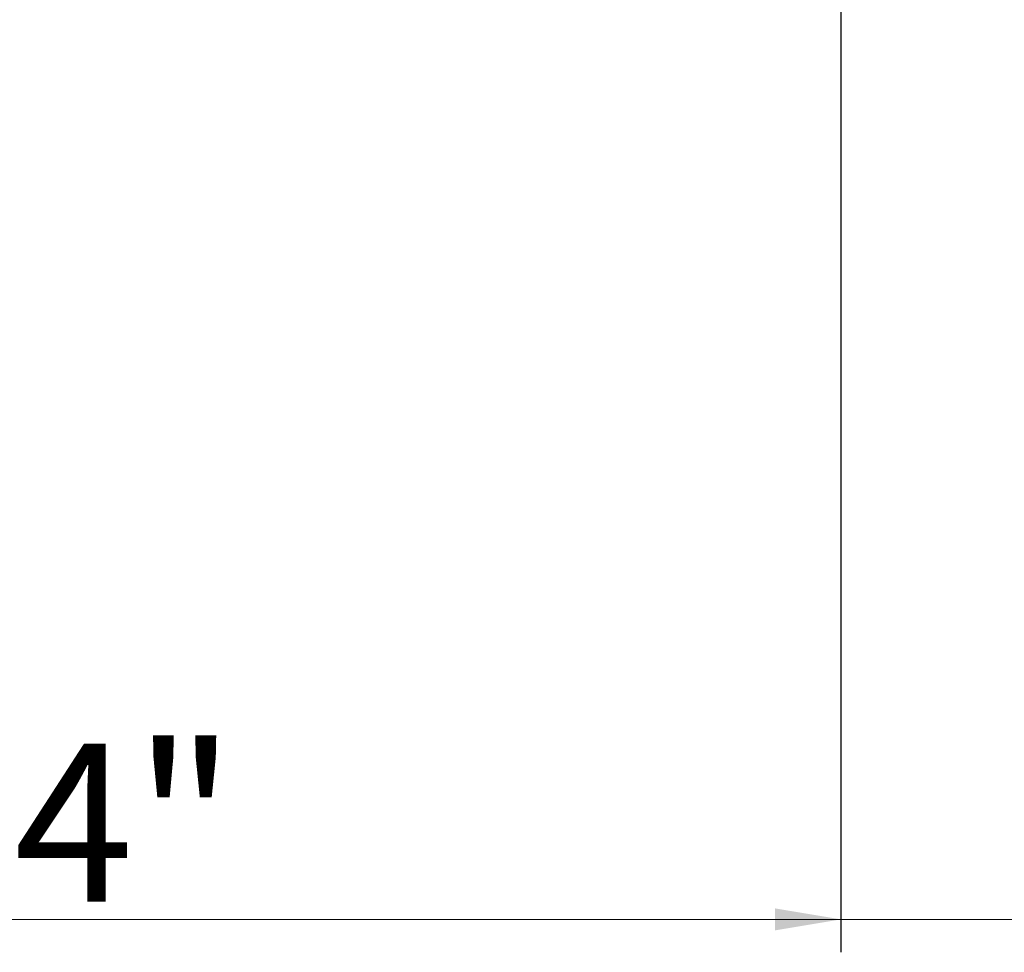
# Model space of a CAD drawing. Units: inches. Extents: x 2696 to 3240, y 1564 to 2310.
# Tile 2 of 76: x 2875 to 2912, y 1569 to 1604. Entities that reach past the tile are written whole.
import ezdxf

# ---------------------------------------------------------------- set-up
doc = ezdxf.new("R2010")
doc.units = ezdxf.units.IN
doc.layers.add('A-ANNO-DIMS', color=3, linetype='Continuous', lineweight=18)
doc.styles.add('TIMES NEW', font='times.ttf')
doc.dimstyles.new('Siddhuu', dxfattribs={"dimtxt": 6, "dimasz": 2.5, "dimexe": 1.25, "dimexo": 0.625, "dimtad": 1, "dimdec": 1, "dimlunit": 4, "dimtxsty": 'TIMES NEW', "dimcen": 2.5, "dimclrd": 256, "dimclre": 1, "dimclrt": 7, "dimadec": 0, "dimazin": 0, "dimtfac": 1, "dimtdec": 1, "dimtmove": 0, "dimatfit": 3, "dimfxl": 1, "dimtolj": 1, "dimlwd": -1, "dimarcsym": 0})

# ---------------------------------------------------------------- blocks, each defined once
blk = doc.blocks.new('*D57')
at = {"layer": 'A-ANNO-DIMS', "color": 1, "lineweight": -2, "transparency": 16777216}
for p, q in [((2754.611, 2018.576), (2754.611, 1568.951)), ((2956.709, 2018.576), (2956.709, 1568.951))]:
    blk.add_line(p, q, dxfattribs=at)
at = {"layer": 'A-ANNO-DIMS', "transparency": 16777216}
blk.add_line((2757.111, 1570.201), (2954.209, 1570.201), dxfattribs=at)
for points in [[(2757.111, 1570.618), (2757.111, 1569.784), (2754.611, 1570.201)], [(2954.209, 1570.618), (2954.209, 1569.784), (2956.709, 1570.201)]]:
    blk.add_solid(points, dxfattribs=at)
at = {"layer": 'Defpoints', "color": 0, "transparency": 16777216}
for p in [(2754.611, 2019.201), (2956.709, 2019.201), (2956.709, 1570.201)]:
    blk.add_point(p, dxfattribs=at)
at = {"layer": 'A-ANNO-DIMS', "color": 7, "transparency": 16777216, "insert": (2855.66, 1573.878), "char_height": 6, "attachment_point": 5, "style": 'TIMES NEW'}
blk.add_mtext('\\A1;16\'-10"', dxfattribs=at)
blk = doc.blocks.new('*D69')
at = {"layer": 'A-ANNO-DIMS', "color": 1, "lineweight": -2, "transparency": 16777216}
for p, q in [((2841.889, 2261.576), (2841.889, 1568.951)), ((2905.91, 2261.576), (2905.91, 1568.951))]:
    blk.add_line(p, q, dxfattribs=at)
at = {"layer": 'A-ANNO-DIMS', "transparency": 16777216}
blk.add_line((2844.389, 1570.201), (2903.41, 1570.201), dxfattribs=at)
for points in [[(2844.389, 1570.618), (2844.389, 1569.784), (2841.889, 1570.201)], [(2903.41, 1570.618), (2903.41, 1569.784), (2905.91, 1570.201)]]:
    blk.add_solid(points, dxfattribs=at)
at = {"layer": 'Defpoints', "color": 0, "transparency": 16777216}
for p in [(2841.889, 2262.201), (2905.91, 2262.201), (2905.91, 1570.201)]:
    blk.add_point(p, dxfattribs=at)
at = {"layer": 'A-ANNO-DIMS', "color": 7, "transparency": 16777216, "insert": (2873.9, 1573.878), "char_height": 6, "attachment_point": 5, "style": 'TIMES NEW'}
blk.add_mtext('\\A1;5\'-4"', dxfattribs=at)

msp = doc.modelspace()

# ---------------------------------------------------------------- dimensions: what is measured, and where the dimension line sits
at = {"layer": 'A-ANNO-DIMS'}
for base, p1, p2, picture, middle in [((2905.91, 1570.201), (2841.889, 2262.201), (2905.91, 2262.201), '*D69', (2873.9, 1573.878)), ((2956.709, 1570.201), (2754.611, 2019.201), (2956.709, 2019.201), '*D57', (2855.66, 1573.878))]:
    dim = msp.add_linear_dim(base=base, p1=p1, p2=p2, dimstyle='Siddhuu', override={"dimdec": 1, "dimlfac": 1, "dimrnd": 0, "dimzin": 1, "dimdsep": 46, "dimlunit": 4, "dimfrac": 2}, dxfattribs=at)
    dim.commit()
    dim.dimension.update_dxf_attribs({"geometry": picture, "text_midpoint": middle})

doc.saveas('drawing.dxf')
